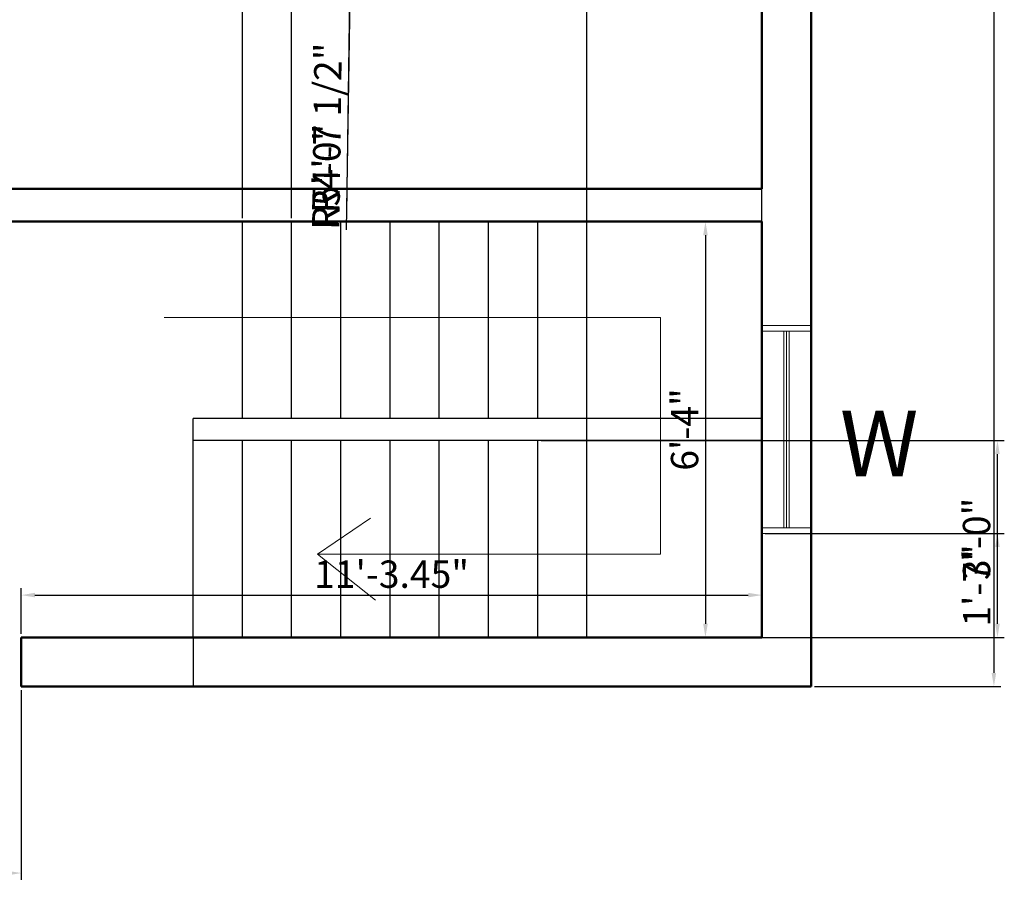
# Model space of a CAD drawing. Units: inches. Extents: x 2050 to 2529, y 1266 to 1968.
# Tile 2 of 5: x 2310 to 2490, y 1266 to 1427. Entities that reach past the tile are written whole.
import ezdxf

# ---------------------------------------------------------------- set-up
doc = ezdxf.new("R2010")
doc.units = ezdxf.units.IN
for name, color, linetype, lineweight in [('A-ANNO-DIMS', 2, 'Continuous', 18), ('A-ANNO-SYMB', 2, 'Continuous', 18), ('A-ANNO-TEXT', 7, 'Continuous', 18), ('A-FLOR-STRS', 7, 'Continuous', 25), ('A-GLAZ', 4, 'Continuous', 18), ('A-WALL', 7, 'Continuous', 50)]:
    doc.layers.add(name, color=color, linetype=linetype, lineweight=lineweight)
doc.styles.get("Standard").update_dxf_attribs({"font": 'arial.ttf'})
doc.dimstyles.new('ISO-25', dxfattribs={"dimtxt": 5, "dimasz": 2.5, "dimexe": 1.25, "dimexo": 0.625, "dimtad": 1, "dimlunit": 3, "dimtxsty": 'Standard', "dimcen": 2.5, "dimadec": 0, "dimazin": 0, "dimtfac": 1, "dimtmove": 0, "dimatfit": 3, "dimfxl": 1, "dimarcsym": 0})

# ---------------------------------------------------------------- blocks, each defined once
blk = doc.blocks.new('*D2')
at = {"layer": 'A-ANNO-DIMS', "color": 0, "lineweight": -2, "transparency": 16777216}
for p, q in [((2454.92, 1844.72), (2488.97, 1844.72)), ((2487.72, 1842.22), (2487.72, 1307.22)), ((2454.92, 1304.72), (2488.97, 1304.72))]:
    blk.add_line(p, q, dxfattribs=at)
at = {"layer": 'A-ANNO-DIMS', "color": 0, "transparency": 16777216}
for points in [[(2487.3, 1842.22), (2488.13, 1842.22), (2487.72, 1844.72)], [(2487.3, 1307.22), (2488.13, 1307.22), (2487.72, 1304.72)]]:
    blk.add_solid(points, dxfattribs=at)
at = {"layer": 'Defpoints', "color": 0, "transparency": 16777216}
for p in [(2454.29, 1844.72), (2454.29, 1304.72), (2487.72, 1304.72)]:
    blk.add_point(p, dxfattribs=at)
at = {"layer": 'A-ANNO-DIMS', "color": 0, "transparency": 16777216, "insert": (2479.46, 1574.72), "char_height": 5, "attachment_point": 5, "rotation": 90}
blk.add_mtext("{\\H3x;45'}", dxfattribs=at)
blk = doc.blocks.new('*D23')
at = {"layer": 'A-ANNO-DIMS', "color": 0, "lineweight": -2, "transparency": 16777216}
for p, q in [((2309.85, 1314.35), (2309.85, 1322.7)), ((2445.29, 1314.35), (2445.29, 1322.7)), ((2312.35, 1321.45), (2442.79, 1321.45))]:
    blk.add_line(p, q, dxfattribs=at)
at = {"layer": 'A-ANNO-DIMS', "color": 0, "transparency": 16777216}
for points in [[(2312.35, 1321.87), (2312.35, 1321.04), (2309.85, 1321.45)], [(2442.79, 1321.87), (2442.79, 1321.04), (2445.29, 1321.45)]]:
    blk.add_solid(points, dxfattribs=at)
at = {"layer": 'Defpoints', "color": 0, "transparency": 16777216}
for p in [(2445.29, 1321.45), (2309.85, 1313.72), (2445.29, 1313.72)]:
    blk.add_point(p, dxfattribs=at)
at = {"layer": 'A-ANNO-DIMS', "color": 0, "transparency": 16777216, "insert": (2377.57, 1324.63), "char_height": 5, "attachment_point": 5}
blk.add_mtext('11\'-3.45"', dxfattribs=at)
blk = doc.blocks.new('*D24')
at = {"layer": 'A-ANNO-DIMS', "color": 0, "lineweight": -2, "transparency": 16777216}
for p, q in [((2444.67, 1389.72), (2433.72, 1389.72)), ((2434.97, 1387.22), (2434.97, 1316.22)), ((2444.67, 1313.72), (2433.72, 1313.72))]:
    blk.add_line(p, q, dxfattribs=at)
at = {"layer": 'A-ANNO-DIMS', "color": 0, "transparency": 16777216}
for points in [[(2434.56, 1387.22), (2435.39, 1387.22), (2434.97, 1389.72)], [(2434.56, 1316.22), (2435.39, 1316.22), (2434.97, 1313.72)]]:
    blk.add_solid(points, dxfattribs=at)
at = {"layer": 'Defpoints', "color": 0, "transparency": 16777216}
for p in [(2445.29, 1389.72), (2434.97, 1313.72), (2445.29, 1313.72)]:
    blk.add_point(p, dxfattribs=at)
at = {"layer": 'A-ANNO-DIMS', "color": 0, "transparency": 16777216, "insert": (2431.8, 1351.72), "char_height": 5, "attachment_point": 5, "rotation": 90}
blk.add_mtext('6\'-4"', dxfattribs=at)
blk = doc.blocks.new('WIN-36IN')
for p, q in [((0, 9), (0, 0)), ((1, 9), (1, 0)), ((37, 9), (37, 0)), ((38, 9), (38, 0)), ((1, 5), (37, 5)), ((1, 4.5), (37, 4.5)), ((1, 4), (37, 4))]:
    blk.add_line(p, q)
blk = doc.blocks.new('*D49')
at = {"layer": 'A-ANNO-DIMS', "color": 0, "lineweight": -2, "transparency": 16777216}
for p, q in [((2269.29, 1304.1), (2269.29, 1269.4)), ((2309.85, 1304.1), (2309.85, 1269.4)), ((2271.79, 1270.65), (2307.35, 1270.65))]:
    blk.add_line(p, q, dxfattribs=at)
at = {"layer": 'A-ANNO-DIMS', "color": 0, "transparency": 16777216}
for points in [[(2271.79, 1271.06), (2271.79, 1270.23), (2269.29, 1270.65)], [(2307.35, 1271.06), (2307.35, 1270.23), (2309.85, 1270.65)]]:
    blk.add_solid(points, dxfattribs=at)
at = {"layer": 'Defpoints', "color": 0, "transparency": 16777216}
for p in [(2269.29, 1304.72), (2309.85, 1304.72), (2309.85, 1270.65)]:
    blk.add_point(p, dxfattribs=at)
at = {"layer": 'A-ANNO-DIMS', "color": 0, "transparency": 16777216, "insert": (2289.57, 1273.86), "char_height": 5, "attachment_point": 5}
blk.add_mtext('3\'-4 1/2"', dxfattribs=at)
blk = doc.blocks.new('*D51')
at = {"layer": 'A-ANNO-DIMS', "color": 0, "lineweight": -2, "transparency": 16777216}
for p, q in [((2413.29, 1314.35), (2413.29, 1907.05)), ((2445.29, 1314.35), (2445.29, 1907.05)), ((2442.79, 1905.8), (2415.79, 1905.8))]:
    blk.add_line(p, q, dxfattribs=at)
at = {"layer": 'A-ANNO-DIMS', "color": 0, "transparency": 16777216}
for points in [[(2415.79, 1906.21), (2415.79, 1905.38), (2413.29, 1905.8)], [(2442.79, 1906.21), (2442.79, 1905.38), (2445.29, 1905.8)]]:
    blk.add_solid(points, dxfattribs=at)
at = {"layer": 'Defpoints', "color": 0, "transparency": 16777216}
for p in [(2413.29, 1905.8), (2413.29, 1313.72), (2445.29, 1313.72)]:
    blk.add_point(p, dxfattribs=at)
at = {"layer": 'A-ANNO-DIMS', "color": 0, "transparency": 16777216, "insert": (2429.29, 1908.97), "char_height": 5, "attachment_point": 5}
blk.add_mtext('2\'-8"', dxfattribs=at)
blk = doc.blocks.new('*D52')
at = {"layer": 'A-ANNO-DIMS', "color": 0, "lineweight": -2, "transparency": 16777216}
for p, q in [((2350.29, 1390.35), (2350.29, 1907.05)), ((2359.29, 1390.35), (2359.29, 1907.05)), ((2352.79, 1905.8), (2356.79, 1905.8)), ((2359.29, 1905.8), (2376.34, 1905.8))]:
    blk.add_line(p, q, dxfattribs=at)
at = {"layer": 'A-ANNO-DIMS', "color": 0, "transparency": 16777216}
for points in [[(2352.79, 1906.21), (2352.79, 1905.38), (2350.29, 1905.8)], [(2356.79, 1906.21), (2356.79, 1905.38), (2359.29, 1905.8)]]:
    blk.add_solid(points, dxfattribs=at)
at = {"layer": 'Defpoints', "color": 0, "transparency": 16777216}
for p in [(2359.29, 1905.8), (2350.29, 1389.72), (2359.29, 1389.72)]:
    blk.add_point(p, dxfattribs=at)
at = {"layer": 'A-ANNO-DIMS', "color": 0, "transparency": 16777216, "insert": (2369.07, 1908.97), "char_height": 5, "attachment_point": 5}
blk.add_mtext('0\'-9"', dxfattribs=at)
blk = doc.blocks.new('*D53')
at = {"layer": 'A-ANNO-DIMS', "color": 0, "lineweight": -2, "transparency": 16777216}
for p, q in [((2404.92, 1349.72), (2489.62, 1349.72)), ((2488.37, 1316.22), (2488.37, 1347.22)), ((2413.92, 1313.72), (2489.62, 1313.72))]:
    blk.add_line(p, q, dxfattribs=at)
at = {"layer": 'A-ANNO-DIMS', "color": 0, "transparency": 16777216}
for points in [[(2487.95, 1347.22), (2488.79, 1347.22), (2488.37, 1349.72)], [(2487.95, 1316.22), (2488.79, 1316.22), (2488.37, 1313.72)]]:
    blk.add_solid(points, dxfattribs=at)
at = {"layer": 'Defpoints', "color": 0, "transparency": 16777216}
for p in [(2404.29, 1349.72), (2488.37, 1349.72), (2413.29, 1313.72)]:
    blk.add_point(p, dxfattribs=at)
at = {"layer": 'A-ANNO-DIMS', "color": 0, "transparency": 16777216, "insert": (2485.19, 1331.72), "char_height": 5, "attachment_point": 5, "rotation": 90}
blk.add_mtext('3\'-0"', dxfattribs=at)
blk = doc.blocks.new('*D73')
at = {"layer": 'A-ANNO-DIMS', "color": 0, "lineweight": -2, "transparency": 16777216}
for p, q in [((2445.92, 1332.72), (2489.62, 1332.72)), ((2488.37, 1316.22), (2488.37, 1330.22)), ((2445.92, 1313.72), (2489.62, 1313.72))]:
    blk.add_line(p, q, dxfattribs=at)
at = {"layer": 'A-ANNO-DIMS', "color": 0, "transparency": 16777216}
for points in [[(2487.95, 1330.22), (2488.79, 1330.22), (2488.37, 1332.72)], [(2487.95, 1316.22), (2488.79, 1316.22), (2488.37, 1313.72)]]:
    blk.add_solid(points, dxfattribs=at)
at = {"layer": 'Defpoints', "color": 0, "transparency": 16777216}
for p in [(2445.29, 1332.72), (2488.37, 1332.72), (2445.29, 1313.72)]:
    blk.add_point(p, dxfattribs=at)
at = {"layer": 'A-ANNO-DIMS', "color": 0, "transparency": 16777216, "insert": (2485.23, 1323.22), "char_height": 5, "attachment_point": 5, "rotation": 90}
blk.add_mtext('1\'-7"', dxfattribs=at)
blk = doc.blocks.new('*D83')
at = {"layer": 'A-ANNO-DIMS', "color": 0, "lineweight": -2, "transparency": 16777216}
for p, q in [((2370.92, 1494.24), (2370.02, 1434)), ((2369.34, 1388.19), (2369.99, 1431.5))]:
    blk.add_line(p, q, dxfattribs=at)
at = {"layer": 'A-ANNO-DIMS', "color": 0, "transparency": 16777216}
blk.add_solid([(2369.57, 1431.51), (2370.4, 1431.49), (2370.02, 1434)], dxfattribs=at)
at = {"layer": 'Defpoints', "color": 0, "transparency": 16777216}
for p in [(2370.92, 1494.24), (2370.02, 1434)]:
    blk.add_point(p, dxfattribs=at)
at = {"layer": 'A-ANNO-DIMS', "color": 0, "transparency": 16777216, "insert": (2366.31, 1397.9), "char_height": 5, "attachment_point": 5, "rotation": 89.147}
blk.add_mtext('R5\'-0"', dxfattribs=at)
blk = doc.blocks.new('*D84')
at = {"layer": 'A-ANNO-DIMS', "color": 0, "lineweight": -2, "transparency": 16777216}
for p, q in [((2370.94, 1495.38), (2370.11, 1440)), ((2369.39, 1391.28), (2370.07, 1437.5))]:
    blk.add_line(p, q, dxfattribs=at)
at = {"layer": 'A-ANNO-DIMS', "color": 0, "transparency": 16777216}
blk.add_solid([(2369.66, 1437.5), (2370.49, 1437.49), (2370.11, 1440)], dxfattribs=at)
at = {"layer": 'Defpoints', "color": 0, "transparency": 16777216}
for p in [(2370.94, 1495.38), (2370.11, 1440)]:
    blk.add_point(p, dxfattribs=at)
at = {"layer": 'A-ANNO-DIMS', "color": 0, "transparency": 16777216, "insert": (2366.41, 1406.82), "char_height": 5, "attachment_point": 5, "rotation": 89.1467}
blk.add_mtext('R4\'-7 1/2"', dxfattribs=at)

msp = doc.modelspace()

# ---------------------------------------------------------------- linework, layer by layer
at = {"layer": 'A-ANNO-SYMB'}
for p, q in [((2335.989, 1372.197), (2426.78, 1372.197)), ((2426.78, 1372.197), (2426.78, 1328.927)), ((2364.002, 1328.927), (2373.738, 1335.484)), ((2426.78, 1328.927), (2364.002, 1328.927)), ((2364.002, 1328.927), (2374.662, 1320.507))]:
    msp.add_line(p, q, dxfattribs=at)
at = {"layer": 'A-FLOR-STRS'}
for p, q in [((2350.295, 1353.72), (2350.295, 1389.72)), ((2359.295, 1353.72), (2359.295, 1389.72)), ((2368.295, 1353.72), (2368.295, 1389.72)), ((2377.295, 1353.72), (2377.295, 1389.72)), ((2386.295, 1353.72), (2386.295, 1389.72)), ((2395.295, 1353.72), (2395.295, 1389.72)), ((2404.295, 1353.72), (2404.295, 1389.72)), ((2413.295, 1313.72), (2413.295, 1389.72)), ((2341.295, 1313.72), (2341.295, 1353.72)), ((2445.295, 1353.72), (2341.295, 1353.72)), ((2445.295, 1349.72), (2341.295, 1349.72)), ((2350.295, 1313.72), (2350.295, 1349.72)), ((2359.295, 1313.72), (2359.295, 1349.72)), ((2368.295, 1313.72), (2368.295, 1349.72)), ((2377.295, 1313.72), (2377.295, 1349.72)), ((2386.295, 1313.72), (2386.295, 1349.72)), ((2395.295, 1313.72), (2395.295, 1349.72)), ((2404.295, 1313.72), (2404.295, 1349.72)), ((2341.295, 1313.72), (2341.295, 1304.72))]:
    msp.add_line(p, q, dxfattribs=at)
at = {"layer": 'A-WALL'}
for p, q in [((2454.295, 1844.72), (2454.295, 1304.72)), ((2445.295, 1685.72), (2445.295, 1395.72)), ((2305.295, 1395.72), (2445.295, 1395.72)), ((2305.295, 1389.72), (2445.295, 1389.72)), ((2445.295, 1389.72), (2445.295, 1313.72)), ((2445.295, 1313.72), (2309.846, 1313.72)), ((2309.846, 1313.72), (2309.846, 1304.72)), ((2454.295, 1304.72), (2309.846, 1304.72))]:
    msp.add_line(p, q, dxfattribs=at)

# ---------------------------------------------------------------- block references
at = {"layer": 'A-GLAZ', "rotation": 269.9999999999998}
msp.add_blockref('WIN-36IN', (2445.294, 1370.72), dxfattribs=at)

# ---------------------------------------------------------------- texts
at = {"layer": 'A-ANNO-TEXT', "insert": (2459.55, 1355.181), "char_height": 12, "attachment_point": 1}
msp.add_mtext_dynamic_manual_height_columns('W', width=471.52273, gutter_width=12.5, heights=[28.462], dxfattribs=at)

# ---------------------------------------------------------------- dimensions: what is measured, and where the dimension line sits
at = {"layer": 'A-ANNO-DIMS'}
for base, p1, p2, override, picture, middle in [((2359.295, 1905.795), (2350.295, 1389.72), (2359.295, 1389.72), {"dimdec": 1, "dimlfac": 1, "dimrnd": 0, "dimzin": 1, "dimdsep": 46, "dimlunit": 4, "dimfrac": 2}, '*D52', (2369.065, 1908.973)), ((2413.295, 1905.795), (2445.295, 1313.72), (2413.295, 1313.72), {"dimdec": 1, "dimlfac": 1, "dimrnd": 0, "dimzin": 1, "dimdsep": 46, "dimlunit": 4, "dimfrac": 2}, '*D51', (2429.295, 1908.973)), ((2445.295, 1321.455), (2309.846, 1313.72), (2445.295, 1313.72), {"dimclrd": 0, "dimclre": 0, "dimclrt": 0}, '*D23', (2377.57, 1324.634)), ((2309.846, 1270.645), (2269.295, 1304.72), (2309.846, 1304.72), {"dimdec": 1, "dimlfac": 1, "dimrnd": 0, "dimzin": 1, "dimdsep": 46, "dimlunit": 4, "dimfrac": 2}, '*D49', (2289.57, 1273.857))]:
    dim = msp.add_linear_dim(base=base, p1=p1, p2=p2, dimstyle='ISO-25', override=override, dxfattribs=at)
    dim.commit()
    dim.dimension.update_dxf_attribs({"geometry": picture, "text_midpoint": middle})
dim = msp.add_linear_dim(base=(2487.716, 1304.72), p1=(2454.295, 1844.72), p2=(2454.295, 1304.72), angle=90, text='{\\H3x;<>}', dimstyle='ISO-25', override={"dimclrd": 0, "dimclre": 0, "dimclrt": 0}, dxfattribs=at)
dim.commit()
dim.dimension.update_dxf_attribs({"geometry": '*D2', "text_midpoint": (2479.463, 1574.72)})
for center, mpoint, picture, middle in [((2370.937, 1495.376), (2370.112, 1439.998), '*D84', (2369.617, 1406.771)), ((2370.92, 1494.242), (2370.023, 1433.999), '*D83', (2369.485, 1397.853))]:
    dim = msp.add_radius_dim(center=center, mpoint=mpoint, dimstyle='ISO-25', override={"dimdec": 1, "dimlfac": 1, "dimrnd": 0, "dimzin": 1, "dimdsep": 46, "dimlunit": 4, "dimfrac": 2}, dxfattribs=at)
    dim.commit()
    dim.dimension.update_dxf_attribs({"geometry": picture, "text_midpoint": middle, "dimtype": 164})
for base, p1, p2, override, picture, middle in [((2434.973, 1313.72), (2445.295, 1389.72), (2445.295, 1313.72), {"dimclrd": 0, "dimclre": 0, "dimclrt": 0}, '*D24', (2431.796, 1351.72)), ((2488.37, 1349.72), (2413.295, 1313.72), (2404.295, 1349.72), {"dimdec": 1, "dimlfac": 1, "dimrnd": 0, "dimzin": 1, "dimdsep": 46, "dimlunit": 4, "dimfrac": 2}, '*D53', (2485.19, 1331.72)), ((2488.37, 1332.72), (2445.295, 1313.72), (2445.295, 1332.72), {"dimdec": 1, "dimlfac": 1, "dimrnd": 0, "dimzin": 1, "dimdsep": 46, "dimlunit": 4, "dimfrac": 2}, '*D73', (2485.234, 1323.22))]:
    dim = msp.add_linear_dim(base=base, p1=p1, p2=p2, angle=90, dimstyle='ISO-25', override=override, dxfattribs=at)
    dim.commit()
    dim.dimension.update_dxf_attribs({"geometry": picture, "text_midpoint": middle})

doc.saveas('drawing.dxf')
